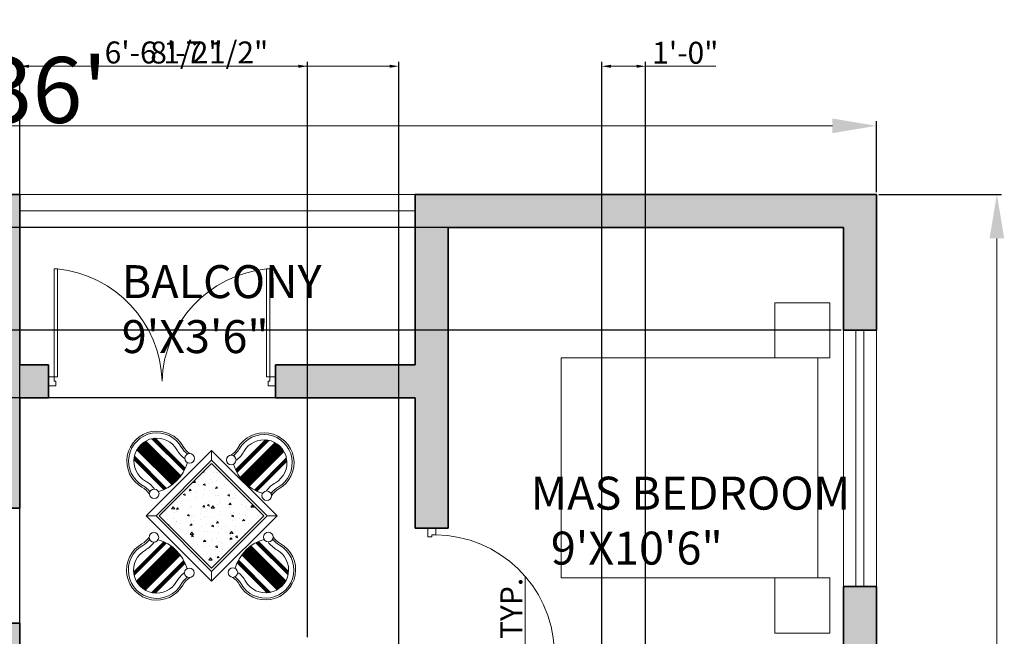
# Model space of a CAD drawing. Units: inches. Extents: x 2696 to 3240, y 1564 to 2310.
# Tile 76 of 76: x 2966 to 3235, y 2142 to 2310. Entities that reach past the tile are written whole.
import ezdxf

# ---------------------------------------------------------------- set-up
doc = ezdxf.new("R2010")
doc.units = ezdxf.units.IN
doc.linetypes.add('ACAD_ISO02W100', pattern=[15, 12, -3])
for name, color, linetype, lineweight in [('A-ANNO-DIMS', 3, 'Continuous', 18), ('A-AREA-IDEN', 7, 'Continuous', 18), ('A-DOOR', 4, 'Continuous', 18), ('A-FLOR-HRAL', 7, 'Continuous', 18), ('A-FURN', 251, 'Continuous', 13), ('A-WALL', 7, 'Continuous', 35), ('A-WALL-OVHD', 7, 'ACAD_ISO02W100', 18), ('A-WALL-PATT', 9, 'Continuous', 13), ('WINDOW', 2, 'Continuous', 18)]:
    doc.layers.add(name, color=color, linetype=linetype, lineweight=lineweight)
doc.styles.add('TIMES NEW', font='times.ttf')
doc.styles.add('YQ_DIM', font='SUPEROS.SHX', dxfattribs={"width": 0.8, "bigfont": 'HZDX.SHX'})
doc.dimstyles.new('Siddhuu', dxfattribs={"dimtxt": 6, "dimasz": 2.5, "dimexe": 1.25, "dimexo": 0.625, "dimtad": 1, "dimdec": 1, "dimlunit": 4, "dimtxsty": 'TIMES NEW', "dimcen": 2.5, "dimclrd": 256, "dimclre": 1, "dimclrt": 7, "dimadec": 0, "dimazin": 0, "dimtfac": 1, "dimtdec": 1, "dimtmove": 0, "dimatfit": 3, "dimfxl": 1, "dimtolj": 1, "dimlwd": -1, "dimarcsym": 0})

# ---------------------------------------------------------------- blocks, each defined once
blk = doc.blocks.new('DR_D01')
for p, q in [((-0.45, 0.93), (-0.42, 0.93)), ((-0.45, 0.03), (-0.45, 0.93)), ((-0.42, 0.03), (-0.42, 0.93)), ((-0.5, 0.03), (-0.42, 0.03)), ((-0.5, 0.03), (-0.5, -0.03)), ((-0.45, 0.03), (-0.45, 0)), ((-0.45, 0), (-0.435, 0)), ((-0.435, 0), (-0.435, -0.03)), ((0.435, 0), (0.435, -0.03)), ((0.45, 0), (0.435, 0)), ((0.45, 0.03), (0.45, 0)), ((0.5, 0.03), (0.45, 0.03)), ((0.5, -0.03), (0.5, 0.03)), ((-0.435, -0.03), (-0.5, -0.03)), ((0.435, -0.03), (0.5, -0.03))]:
    blk.add_line(p, q)
blk.add_arc((-0.4602, 0.0206), 0.9103, 0.59152, 87.46644)
blk = doc.blocks.new('DR_D02')
for p, q in [((-0.46, 0.4948), (-0.475, 0.4948)), ((-0.475, 0.02), (-0.475, 0.4948)), ((-0.46, 0.02), (-0.46, 0.495)), ((0.46, 0.02), (0.46, 0.495)), ((0.46, 0.4948), (0.475, 0.4948)), ((0.475, 0.02), (0.475, 0.4948)), ((-0.46, 0.02), (-0.5, 0.02)), ((-0.5, 0.02), (-0.5, -0.02)), ((-0.475, 0.02), (-0.475, 0)), ((-0.475, 0), (-0.4675, 0)), ((-0.4675, 0), (-0.4675, -0.02)), ((0.46, 0.02), (0.5, 0.02)), ((0.4675, 0), (0.4675, -0.02)), ((0.475, 0), (0.4675, 0)), ((0.475, 0.02), (0.475, 0)), ((0.5, 0.02), (0.5, -0.02)), ((-0.4675, -0.02), (-0.5, -0.02)), ((0.4675, -0.02), (0.5, -0.02))]:
    blk.add_line(p, q)
for centre, start, end in [((-0.5121, -0.0149), 1.6619, 84.1677), ((0.5121, -0.0149), 95.8323, 178.3381)]:
    blk.add_arc(centre, 0.5123, start, end)
blk = doc.blocks.new('WD_WIN4')
for p, q in [((-0.5, 0.5), (0.5, 0.5)), ((-0.5, 0.12), (0.5, 0.12)), ((-0.5, -0.12), (0.5, -0.12)), ((-0.5, -0.5), (0.5, -0.5))]:
    blk.add_line(p, q)
blk = doc.blocks.new('*D9')
at = {"layer": 'A-ANNO-DIMS', "color": 0, "lineweight": -2, "transparency": 16777216}
for p, q in [((2745.61, 2262.83), (2745.61, 2282.19)), ((3199.61, 2262.83), (3199.61, 2282.19))]:
    blk.add_line(p, q, dxfattribs=at)
at = {"layer": 'A-ANNO-DIMS', "color": 0, "transparency": 16777216}
blk.add_line((2757.61, 2280.94), (3187.61, 2280.94), dxfattribs=at)
for points in [[(2757.61, 2282.94), (2757.61, 2278.94), (2745.61, 2280.94)], [(3187.61, 2282.94), (3187.61, 2278.94), (3199.61, 2280.94)]]:
    blk.add_solid(points, dxfattribs=at)
at = {"layer": 'Defpoints', "color": 0, "transparency": 16777216}
for p in [(3199.61, 2280.94), (2745.61, 2262.2), (3199.61, 2262.2)]:
    blk.add_point(p, dxfattribs=at)
at = {"layer": 'A-ANNO-DIMS', "color": 0, "transparency": 16777216, "insert": (2972.61, 2290.72), "char_height": 18, "attachment_point": 5, "style": 'TIMES NEW'}
blk.add_mtext("\\A1;36'", dxfattribs=at)
blk = doc.blocks.new('*D10')
at = {"layer": 'A-ANNO-DIMS', "color": 0, "lineweight": -2, "transparency": 16777216}
for p, q in [((3200.24, 2262.2), (3233.75, 2262.2)), ((3200.24, 1605.2), (3233.75, 1605.2))]:
    blk.add_line(p, q, dxfattribs=at)
at = {"layer": 'A-ANNO-DIMS', "color": 0, "transparency": 16777216}
blk.add_line((3232.5, 2250.2), (3232.5, 1617.2), dxfattribs=at)
for points in [[(3230.5, 2250.2), (3234.5, 2250.2), (3232.5, 2262.2)], [(3230.5, 1617.2), (3234.5, 1617.2), (3232.5, 1605.2)]]:
    blk.add_solid(points, dxfattribs=at)
at = {"layer": 'Defpoints', "color": 0, "transparency": 16777216}
for p in [(3199.61, 2262.2), (3199.61, 1605.2), (3232.5, 1605.2)]:
    blk.add_point(p, dxfattribs=at)
at = {"layer": 'A-ANNO-DIMS', "color": 0, "transparency": 16777216, "insert": (3222.71, 1933.7), "char_height": 18, "attachment_point": 5, "rotation": 90, "style": 'TIMES NEW'}
blk.add_mtext("\\A1;54'", dxfattribs=at)
blk = doc.blocks.new('DINING-SET-4')
h = blk.add_hatch()
h.set_pattern_fill('AR-CONC,_O', color=256, scale=0.03156, angle=135)
h.set_pattern_definition([(185, (694.1166, -47.9622), (-3.709933, 4.421326), [0.60121, -6.613307]), (130, (694.1166, -47.962), (-3.47714, -5.050095), [0.48097, -5.290645]), (235.451, (693.8074, -47.594), (-7.187067, -0.628735), [0.51095, -5.620443]), (181.1842, (692.983, -49.096), (-5.11118, 6.98761), [0.90181, -9.91996]), (231.6356, (692.557, -48.514), (-10.81945, -0.22364), [0.76642, -8.43066]), (126.184, (692.983, -49.096), (-10.81945, -0.22362), [0.72145, -7.93597]), (156, (692.6995, -48.2457), (-1.10128, 5.66559), [0.60121, -6.613307]), (101, (692.6995, -48.2457), (-5.48951, -2.73116), [0.48097, -5.290645]), (206.4514, (692.608, -47.7735), (-6.590787, 2.93441), [0.51095, -5.620443]), (172.5, (694.1166, -47.9622), (-1.955854, -1.8180035), [0, -5.226516, 0, -5.370807, 0, -5.310686]), (142.5, (694.1166, -47.9622), (-3.726774, -0.744482), [0, -3.062161, 0, -5.106274, 0, -2.024073]), (102.5, (695.3806, -49.2263), (-2.8979947, 3.15368), [0, -2.004032, 0, -6.25258, 0, -8.296694]), (92.5, (695.9475, -49.793), (-3.873065, 2.73823), [0, -2.605242, 0, -4.152355, 0, -5.891855])])
h.paths.add_polyline_path([(23.22, 8.74), (37.5, 23.02), (23.22, 37.31), (8.94, 23.02)])
for p, q in [((14.34, 33.33), (4.62, 43.06)), ((14.5, 33.52), (4.82, 43.2)), ((14.65, 33.71), (5.03, 43.33)), ((14.79, 33.91), (5.25, 43.45)), ((15.69, 35.33), (6.93, 44.09)), ((15.81, 35.56), (7.22, 44.15)), ((15.92, 35.79), (7.52, 44.19)), ((16.03, 36.02), (7.83, 44.22)), ((29.77, 35.57), (37.97, 43.77)), ((29.88, 35.34), (38.28, 43.74)), ((29.99, 35.11), (38.58, 43.7)), ((30.11, 34.88), (38.86, 43.64)), ((12.42, 31.5), (2.84, 41.08)), ((12.61, 31.65), (2.97, 41.3)), ((12.8, 31.8), (3.1, 41.5)), ((12.99, 31.96), (3.24, 41.7)), ((13.17, 32.12), (3.39, 41.89)), ((13.35, 32.28), (3.55, 42.08)), ((13.52, 32.45), (3.71, 42.26)), ((13.69, 32.62), (3.88, 42.43)), ((13.86, 32.79), (4.05, 42.6)), ((14.03, 32.97), (4.24, 42.76)), ((14.19, 33.15), (4.42, 42.91)), ((23.22, 38.2), (23.22, 40.88)), ((31, 33.46), (40.55, 43.01)), ((31.15, 33.26), (40.76, 42.88)), ((31.3, 33.07), (40.97, 42.75)), ((31.45, 32.88), (41.18, 42.61)), ((31.61, 32.7), (41.37, 42.46)), ((31.77, 32.52), (41.56, 42.31)), ((31.93, 32.34), (41.74, 42.15)), ((32.1, 32.17), (41.92, 41.98)), ((32.27, 32), (42.09, 41.81)), ((32.45, 31.83), (42.25, 41.63)), ((32.63, 31.67), (42.4, 41.45)), ((32.81, 31.51), (42.55, 41.25)), ((32.99, 31.35), (42.69, 41.05)), ((33.18, 31.2), (42.83, 40.85)), ((33.38, 31.05), (42.96, 40.63)), ((10.21, 30.19), (2.02, 38.38)), ((10.44, 30.3), (2.05, 38.7)), ((10.67, 30.41), (2.09, 39)), ((10.9, 30.53), (2.15, 39.28)), ((34.9, 30.08), (43.65, 38.83)), ((35.12, 29.96), (43.7, 38.55)), ((35.35, 29.85), (43.75, 38.25)), ((35.58, 29.74), (43.78, 37.94)), ((8.05, 23.02), (5.37, 23.02)), ((38.4, 23.02), (41.07, 23.02)), ((10.15, 15.95), (1.95, 7.75)), ((10.38, 15.84), (1.98, 7.44)), ((10.61, 15.73), (2.02, 7.14)), ((10.84, 15.61), (2.08, 6.86)), ((12.26, 14.72), (2.71, 5.17)), ((12.46, 14.57), (2.84, 4.95)), ((12.65, 14.42), (2.97, 4.75)), ((12.83, 14.27), (3.11, 4.54)), ((13.02, 14.11), (3.26, 4.35)), ((13.2, 13.95), (3.41, 4.16)), ((13.38, 13.78), (3.57, 3.98)), ((13.55, 13.62), (3.74, 3.8)), ((13.72, 13.45), (3.91, 3.63)), ((32.44, 13.53), (42.25, 3.72)), ((32.61, 13.7), (42.42, 3.89)), ((32.78, 13.87), (42.59, 4.06)), ((32.96, 14.03), (42.75, 4.24)), ((33.14, 14.19), (42.9, 4.43)), ((33.33, 14.35), (43.05, 4.63)), ((33.51, 14.5), (43.19, 4.83)), ((33.7, 14.65), (43.32, 5.04)), ((33.9, 14.8), (43.45, 5.25)), ((35.33, 15.7), (44.08, 6.94)), ((35.55, 15.81), (44.14, 7.23)), ((35.78, 15.93), (44.18, 7.52)), ((36.01, 16.03), (44.21, 7.83)), ((13.89, 13.27), (4.09, 3.47)), ((14.05, 13.09), (4.27, 3.32)), ((14.21, 12.91), (4.47, 3.17)), ((14.36, 12.72), (4.67, 3.03)), ((14.52, 12.54), (4.87, 2.89)), ((14.67, 12.34), (5.08, 2.76)), ((15.64, 10.82), (6.89, 2.07)), ((30.52, 10.91), (39.27, 2.15)), ((31.49, 12.43), (41.08, 2.85)), ((31.64, 12.62), (41.29, 2.97)), ((31.8, 12.81), (41.5, 3.11)), ((31.95, 12.99), (41.69, 3.25)), ((32.11, 13.18), (41.89, 3.4)), ((32.27, 13.35), (42.07, 3.55)), ((15.75, 10.6), (7.17, 2.02)), ((15.87, 10.37), (7.47, 1.97)), ((15.98, 10.14), (7.78, 1.94)), ((30.18, 10.22), (38.38, 2.03)), ((30.29, 10.45), (38.69, 2.06)), ((30.41, 10.68), (38.99, 2.1)), ((23.22, 7.85), (23.22, 5.17))]:
    blk.add_line(p, q)
for points in [[(41.07, 23.02), (23.22, 40.88), (5.37, 23.02), (23.22, 5.17)], [(38.4, 23.02), (23.22, 38.2), (8.05, 23.02), (23.22, 7.85)], [(37.5, 23.02), (23.22, 37.31), (8.94, 23.02), (23.22, 8.74)]]:
    blk.add_lwpolyline(points, close=True)
for centre in [(17.23, 38.71), (28.57, 38.26), (7.55, 29.03), (38.27, 28.51), (7.46, 17.15), (38.7, 17.23), (17.14, 7.47), (29.03, 7.55)]:
    blk.add_circle(centre, 1.31)
for centre, radius, start, end in [((8.28, 37.96), 8.21, 29.1881, 240.1532), ((37.51, 37.51), 8.21, 299.8468, 150.8119), ((8.28, 37.96), 7.72, 29.1881, 240.1532), ((8.28, 37.96), 6.28, 29.2752, 240.1505), ((37.51, 37.51), 7.72, 299.8468, 150.8119), ((37.51, 37.51), 6.28, 299.8495, 150.7248), ((20.45, 44.88), 7.72, 209.8594, 234.0675), ((20.45, 44.88), 6.28, 210.1015, 232.6572), ((20.45, 44.88), 5.79, 210.1015, 236.9513), ((25.34, 44.43), 5.79, 303.0487, 329.8985), ((25.34, 44.43), 6.28, 307.3428, 329.8985), ((25.34, 44.43), 7.72, 305.9325, 330.1406), ((5.4, 40.81), 11.66, 286.5158, 343.8317), ((40.4, 40.36), 11.66, 196.1683, 253.4842), ((1.37, 25.79), 7.72, 36.1055, 60.6071), ((1.37, 25.79), 5.79, 32.6748, 60.7093), ((1.37, 25.79), 6.28, 37.2611, 60.7093), ((44.43, 25.34), 7.72, 119.3929, 143.8945), ((44.43, 25.34), 6.28, 119.2907, 142.7389), ((44.43, 25.34), 5.79, 119.2907, 147.3252), ((1.29, 20.38), 5.79, 300.1015, 326.9513), ((1.29, 20.38), 6.28, 300.1015, 322.6572), ((5.36, 5.32), 11.66, 16.5158, 73.8317), ((40.8, 5.4), 11.66, 106.1683, 163.4842), ((44.87, 20.46), 6.28, 217.3428, 239.8985), ((44.87, 20.46), 5.79, 213.0487, 239.8985), ((8.21, 8.21), 8.21, 119.1881, 330.1532), ((8.21, 8.21), 7.72, 119.1881, 330.1532), ((8.21, 8.21), 6.28, 119.2752, 330.1505), ((1.29, 20.38), 7.72, 299.8594, 324.0675), ((37.95, 8.29), 8.21, 209.8468, 60.8119), ((37.95, 8.29), 7.72, 209.8468, 60.8119), ((37.95, 8.29), 6.28, 209.8495, 60.7248), ((44.87, 20.46), 7.72, 215.9325, 240.1406), ((20.38, 1.29), 7.72, 126.1055, 150.6071), ((20.38, 1.29), 6.28, 127.2611, 150.7093), ((20.38, 1.29), 5.79, 122.6748, 150.7093), ((25.78, 1.37), 5.79, 29.2907, 57.3252), ((25.78, 1.37), 6.28, 29.2907, 52.7389), ((25.78, 1.37), 7.72, 29.3929, 53.8945)]:
    blk.add_arc(centre, radius, start, end)
blk = doc.blocks.new('BED-DOUBLE-WITH-NIGHTSTANDS')
for points in [[(0, 75.13), (0, 90.16), (15.03, 90.16), (15.03, 75.13)], [(3.28, 15.03), (3.28, 75.13), (73.4, 75.13), (73.4, 15.03)], [(0, 15.03), (0, 0), (15.03, 0), (15.03, 15.03)]]:
    blk.add_lwpolyline(points, close=True)
blk = doc.blocks.new('*D39')
at = {"layer": 'A-ANNO-DIMS', "transparency": 16777216}
for p, q in [((3103.69, 2104.03), (3103.69, 2157.84)), ((3103.69, 2091.94), (3103.69, 2101.53))]:
    blk.add_line(p, q, dxfattribs=at)
at = {"layer": 'A-ANNO-DIMS', "color": 1, "lineweight": -2, "transparency": 16777216}
for p, q in [((3105.99, 2104.03), (3102.44, 2104.03)), ((3105.99, 2089.44), (3102.44, 2089.44))]:
    blk.add_line(p, q, dxfattribs=at)
at = {"layer": 'A-ANNO-DIMS', "transparency": 16777216}
for points in [[(3103.28, 2101.53), (3104.11, 2101.53), (3103.69, 2104.03)], [(3103.28, 2091.94), (3104.11, 2091.94), (3103.69, 2089.44)]]:
    blk.add_solid(points, dxfattribs=at)
at = {"layer": 'Defpoints', "color": 0, "transparency": 16777216}
for p in [(3103.69, 2104.03), (3106.61, 2104.03), (3106.61, 2089.44)]:
    blk.add_point(p, dxfattribs=at)
at = {"layer": 'A-ANNO-DIMS', "color": 7, "transparency": 16777216, "insert": (3099.93, 2132.19), "char_height": 6, "attachment_point": 5, "rotation": 90, "style": 'TIMES NEW'}
blk.add_mtext('\\A1;1\'-2 1/2" TYP.', dxfattribs=at)
blk = doc.blocks.new('*D54')
at = {"layer": 'A-ANNO-DIMS', "color": 1, "lineweight": -2, "transparency": 16777216}
for p, q in [((3124.61, 1893.83), (3124.61, 2298.45)), ((3136.61, 1893.83), (3136.61, 2298.45))]:
    blk.add_line(p, q, dxfattribs=at)
at = {"layer": 'A-ANNO-DIMS', "transparency": 16777216}
for p, q in [((3127.11, 2297.2), (3134.11, 2297.2)), ((3136.61, 2297.2), (3155.76, 2297.2))]:
    blk.add_line(p, q, dxfattribs=at)
for points in [[(3127.11, 2297.62), (3127.11, 2296.78), (3124.61, 2297.2)], [(3134.11, 2297.62), (3134.11, 2296.78), (3136.61, 2297.2)]]:
    blk.add_solid(points, dxfattribs=at)
at = {"layer": 'Defpoints', "color": 0, "transparency": 16777216}
for p in [(3136.61, 2297.2), (3124.61, 1893.2), (3136.61, 1893.2)]:
    blk.add_point(p, dxfattribs=at)
at = {"layer": 'A-ANNO-DIMS', "color": 7, "transparency": 16777216, "insert": (3147.43, 2300.88), "char_height": 6, "attachment_point": 5, "style": 'TIMES NEW'}
blk.add_mtext('\\A1;1\'-0"', dxfattribs=at)
blk = doc.blocks.new('*D61')
at = {"layer": 'A-ANNO-DIMS', "color": 1, "lineweight": -2, "transparency": 16777216}
for p, q in [((2965.71, 2141.33), (2965.71, 2298.45)), ((3044.3, 2141.33), (3044.3, 2298.45))]:
    blk.add_line(p, q, dxfattribs=at)
at = {"layer": 'A-ANNO-DIMS', "transparency": 16777216}
blk.add_line((2968.21, 2297.2), (3041.8, 2297.2), dxfattribs=at)
for points in [[(2968.21, 2297.62), (2968.21, 2296.78), (2965.71, 2297.2)], [(3041.8, 2297.62), (3041.8, 2296.78), (3044.3, 2297.2)]]:
    blk.add_solid(points, dxfattribs=at)
at = {"layer": 'Defpoints', "color": 0, "transparency": 16777216}
for p in [(3044.3, 2297.2), (2965.71, 2140.7), (3044.3, 2140.7)]:
    blk.add_point(p, dxfattribs=at)
at = {"layer": 'A-ANNO-DIMS', "color": 7, "transparency": 16777216, "insert": (3005.01, 2300.96), "char_height": 6, "attachment_point": 5, "style": 'TIMES NEW'}
blk.add_mtext('\\A1;6\'-6 1/2"', dxfattribs=at)
blk = doc.blocks.new('*D63')
at = {"layer": 'A-ANNO-DIMS', "color": 1, "lineweight": -2, "transparency": 16777216}
for p, q in [((2965.71, 1989.83), (2965.71, 2298.45)), ((3069.21, 1989.83), (3069.21, 2298.45))]:
    blk.add_line(p, q, dxfattribs=at)
at = {"layer": 'A-ANNO-DIMS', "transparency": 16777216}
blk.add_line((2968.21, 2297.2), (3066.71, 2297.2), dxfattribs=at)
for points in [[(2968.21, 2297.62), (2968.21, 2296.78), (2965.71, 2297.2)], [(3066.71, 2297.62), (3066.71, 2296.78), (3069.21, 2297.2)]]:
    blk.add_solid(points, dxfattribs=at)
at = {"layer": 'Defpoints', "color": 0, "transparency": 16777216}
for p in [(3069.21, 2297.2), (2965.71, 1989.2), (3069.21, 1989.2)]:
    blk.add_point(p, dxfattribs=at)
at = {"layer": 'A-ANNO-DIMS', "color": 7, "transparency": 16777216, "insert": (3017.46, 2300.96), "char_height": 6, "attachment_point": 5, "style": 'TIMES NEW'}
blk.add_mtext('\\A1;8\'-7 1/2"', dxfattribs=at)
blk = doc.blocks.new('*D64')
at = {"layer": 'A-ANNO-DIMS', "color": 1, "lineweight": -2, "transparency": 16777216}
for p, q in [((3073.08, 2206.7), (2709.36, 2206.7)), ((3068.58, 1989.2), (2709.36, 1989.2))]:
    blk.add_line(p, q, dxfattribs=at)
at = {"layer": 'A-ANNO-DIMS', "transparency": 16777216}
blk.add_line((2710.61, 1991.7), (2710.61, 2204.2), dxfattribs=at)
for points in [[(2710.19, 2204.2), (2711.03, 2204.2), (2710.61, 2206.7)], [(2710.19, 1991.7), (2711.03, 1991.7), (2710.61, 1989.2)]]:
    blk.add_solid(points, dxfattribs=at)
at = {"layer": 'Defpoints', "color": 0, "transparency": 16777216}
for p in [(2710.61, 2206.7), (3073.71, 2206.7), (3069.21, 1989.2)]:
    blk.add_point(p, dxfattribs=at)
at = {"layer": 'A-ANNO-DIMS', "color": 7, "transparency": 16777216, "insert": (2706.85, 2097.95), "char_height": 6, "attachment_point": 5, "rotation": 90, "style": 'TIMES NEW'}
blk.add_mtext('\\A1;18\'-1 1/2"', dxfattribs=at)
blk = doc.blocks.new('*D76')
at = {"layer": 'A-ANNO-DIMS', "color": 1, "lineweight": -2, "transparency": 16777216}
for p, q in [((3189.99, 2253.2), (2709.36, 2253.2)), ((3189.99, 2225.2), (2709.36, 2225.2))]:
    blk.add_line(p, q, dxfattribs=at)
at = {"layer": 'A-ANNO-DIMS', "transparency": 16777216}
blk.add_line((2710.61, 2250.7), (2710.61, 2227.7), dxfattribs=at)
for points in [[(2710.19, 2250.7), (2711.03, 2250.7), (2710.61, 2253.2)], [(2710.19, 2227.7), (2711.03, 2227.7), (2710.61, 2225.2)]]:
    blk.add_solid(points, dxfattribs=at)
at = {"layer": 'Defpoints', "color": 0, "transparency": 16777216}
for p in [(3190.61, 2253.2), (2710.61, 2225.2), (3190.61, 2225.2)]:
    blk.add_point(p, dxfattribs=at)
at = {"layer": 'A-ANNO-DIMS', "color": 7, "transparency": 16777216, "insert": (2706.99, 2239.2), "char_height": 6, "attachment_point": 5, "rotation": 90, "style": 'TIMES NEW'}
blk.add_mtext('\\A1;2\'-4"', dxfattribs=at)

msp = doc.modelspace()

# ---------------------------------------------------------------- hatches: boundary and pattern name
at = {"layer": 'A-WALL-PATT', "transparency": 33554556}
h = msp.add_hatch(color=256, dxfattribs=at)
h.dxf.hatch_style = 1
h.paths.add_polyline_path([(2879.11, 2253.2), (2905.91, 2253.2), (2905.91, 2262.2), (2841.89, 2262.2), (2841.89, 2253.2), (2870.11, 2253.2), (2870.11, 2176.6), (2965.71, 2176.6), (2965.71, 2206.7), (2973.58, 2206.7), (2973.58, 2215.7), (2965.71, 2215.7), (2965.71, 2262.2), (2929.91, 2262.2), (2929.91, 2253.2), (2956.71, 2253.2), (2956.71, 2185.6), (2879.11, 2185.6)])
h.paths.add_polyline_path([(2782.83, 2262.2), (2745.61, 2262.2), (2745.61, 2228.73), (2754.61, 2228.73), (2754.61, 2253.2), (2782.83, 2253.2)])
h.paths.add_polyline_path([(2754.61, 2136.2), (2965.71, 2136.2), (2965.71, 2145.2), (2879.11, 2145.2), (2879.11, 2147.07), (2877.34, 2147.07), (2870.11, 2147.07), (2870.11, 2145.2), (2754.61, 2145.2), (2754.61, 2169.67), (2745.61, 2169.67), (2745.61, 2000.2), (2754.61, 2000.2), (2754.61, 2019.2), (2849.08, 2019.2), (2849.08, 2023.7), (2841.21, 2023.7), (2841.21, 2051.83), (2836.71, 2051.83), (2836.71, 2023.7), (2754.61, 2023.7), (2754.61, 2091.2), (2836.71, 2091.2), (2836.71, 2087.83), (2841.21, 2087.83), (2841.21, 2095.7), (2754.61, 2095.7)])
h.paths.add_polyline_path([(2965.71, 2136.2), (2956.71, 2136.2), (2956.71, 2023.7), (2885.08, 2023.7), (2885.08, 2019.2), (2956.71, 2019.2), (2956.71, 1950.58), (2965.71, 1950.58), (2965.71, 1980.2), (2973.58, 1980.2), (2973.58, 1989.2), (2965.71, 1989.2)])
h.paths.add_polyline_path([(2754.61, 1906.7), (2880.21, 1906.7), (2884.71, 1906.7), (2956.71, 1906.7), (2956.71, 1792.7), (2944.71, 1792.7), (2944.71, 1783.7), (2956.71, 1783.7), (2956.71, 1740.2), (2884.71, 1740.2), (2884.71, 1783.7), (2896.71, 1783.7), (2896.71, 1792.7), (2884.71, 1792.7), (2884.71, 1846.7), (2880.21, 1846.7), (2880.21, 1740.2), (2754.61, 1740.2), (2754.61, 1777.2), (2745.61, 1777.2), (2745.61, 1692.7), (2754.61, 1692.7), (2754.61, 1731.2), (2956.71, 1731.2), (2956.71, 1723.33), (2965.71, 1723.33), (2965.71, 1884.2), (2973.58, 1884.2), (2973.58, 1893.2), (2965.71, 1893.2), (2965.71, 1914.58), (2956.71, 1914.58), (2956.71, 1911.2), (2754.61, 1911.2), (2754.61, 1930.2), (2745.61, 1930.2), (2745.61, 1817.2), (2754.61, 1817.2), (2754.61, 1854.2), (2826.61, 1854.2), (2826.61, 1868.83), (2822.11, 1868.83), (2822.11, 1858.7), (2754.61, 1858.7)])
h.paths.add_polyline_path([(2965.71, 1656.2), (3008.24, 1656.2), (3008.24, 1665.2), (2965.71, 1665.2), (2965.71, 1693.33), (2956.71, 1693.33), (2956.71, 1686.2), (2934.58, 1686.2), (2934.58, 1681.7), (2956.71, 1681.7), (2956.71, 1614.2), (2896.71, 1614.2), (2896.71, 1681.7), (2904.58, 1681.7), (2904.58, 1686.2), (2892.21, 1686.2), (2892.21, 1614.2), (2858.41, 1614.2), (2858.41, 1605.2), (2965.71, 1605.2)])
h.paths.add_polyline_path([(2788.41, 1614.2), (2754.61, 1614.2), (2754.61, 1652.7), (2745.61, 1652.7), (2745.61, 1605.2), (2788.41, 1605.2)])
h.paths.add_polyline_path([(3199.61, 1633.05), (3190.61, 1633.05), (3190.61, 1614.2), (3082.61, 1614.2), (3082.61, 1665.2), (3070.24, 1665.2), (3070.24, 1656.2), (3078.11, 1656.2), (3078.11, 1605.2), (3199.61, 1605.2)])
h.paths.add_polyline_path([(3199.61, 1702.05), (3190.61, 1702.05), (3190.61, 1699.7), (3106.61, 1699.7), (3106.61, 1747.7), (3190.61, 1747.7), (3190.61, 1752.2), (3082.61, 1752.2), (3082.61, 1760.08), (3078.11, 1760.08), (3078.11, 1747.7), (3102.11, 1747.7), (3102.11, 1699.7), (3078.11, 1699.7), (3078.11, 1695.2), (3190.61, 1695.2), (3190.61, 1676.35), (3199.61, 1676.35)])
h.paths.add_polyline_path([(3199.61, 1783.2), (3190.61, 1783.2), (3190.61, 1745.35), (3199.61, 1745.35)])
h.paths.add_polyline_path([(3082.61, 1884.2), (3190.61, 1884.2), (3190.61, 1853.2), (3199.61, 1853.2), (3199.61, 1901.7), (3190.61, 1901.7), (3190.61, 1893.2), (3005.58, 1893.2), (3005.58, 1891.28), (3005.58, 1884.2), (3078.11, 1884.2), (3078.11, 1792.08), (3082.61, 1792.08)])
h.paths.add_polyline_path([(3199.61, 1994.7), (3190.61, 1994.7), (3190.61, 1989.2), (3073.71, 1989.2), (3073.71, 2034.2), (3069.21, 2034.2), (3069.21, 1989.2), (3005.58, 1989.2), (3005.58, 1980.2), (3190.61, 1980.2), (3190.61, 1971.7), (3199.61, 1971.7)])
h.paths.add_polyline_path([(3199.61, 2155.2), (3190.61, 2155.2), (3190.61, 2064.7), (3199.61, 2064.7)])
h.paths.add_polyline_path([(3190.61, 2074.7), (3106.61, 2074.7), (3106.61, 2122.7), (3190.61, 2122.7), (3190.61, 2127.2), (3082.71, 2127.2), (3082.71, 2135.08), (3073.71, 2135.08), (3073.71, 2122.7), (3102.11, 2122.7), (3102.11, 2074.7), (3069.21, 2074.7), (3069.21, 2070.2), (3190.61, 2070.2)])
h.paths.add_polyline_path([(3082.71, 2253.2), (3190.61, 2253.2), (3190.61, 2225.2), (3199.61, 2225.2), (3199.61, 2262.2), (3073.71, 2262.2), (3073.71, 2215.7), (3035.58, 2215.7), (3035.58, 2206.7), (3073.71, 2206.7), (3073.71, 2171.08), (3082.71, 2171.08)])

# ---------------------------------------------------------------- linework, layer by layer
at = {"layer": 'A-FLOR-HRAL'}
for p, q in [((3073.71, 2262.2), (2965.71, 2262.2)), ((3073.71, 2257.7), (2965.71, 2257.7))]:
    msp.add_line(p, q, dxfattribs=at)
at = {"layer": 'A-WALL'}
for p, q in [((2929.91, 2262.2), (2965.71, 2262.2)), ((2965.71, 2215.7), (2965.71, 2262.2)), ((3073.71, 2262.2), (3199.61, 2262.2)), ((3073.71, 2215.7), (3073.71, 2262.2)), ((3199.61, 2225.2), (3199.61, 2262.2)), ((3082.71, 2253.2), (3190.61, 2253.2)), ((3082.71, 2171.08), (3082.71, 2253.2)), ((3190.61, 2225.2), (3190.61, 2253.2)), ((3190.61, 2225.2), (3199.61, 2225.2)), ((2973.58, 2215.7), (2965.71, 2215.7)), ((2973.58, 2206.7), (2973.58, 2215.7)), ((3073.71, 2215.7), (3035.58, 2215.7)), ((3035.58, 2206.7), (3035.58, 2215.7)), ((2965.71, 2176.6), (2965.71, 2206.7)), ((2973.58, 2206.7), (2965.71, 2206.7)), ((3073.71, 2206.7), (3035.58, 2206.7)), ((3073.71, 2171.08), (3073.71, 2206.7)), ((2870.11, 2176.6), (2965.71, 2176.6)), ((3082.71, 2171.08), (3073.71, 2171.08)), ((3190.61, 2155.2), (3199.61, 2155.2)), ((3190.61, 2064.7), (3190.61, 2155.2)), ((3199.61, 2064.7), (3199.61, 2155.2)), ((2879.11, 2145.2), (2965.71, 2145.2)), ((2965.71, 2145.2), (2965.71, 2136.2))]:
    msp.add_line(p, q, dxfattribs=at)
at = {"layer": 'A-WALL-OVHD'}
msp.add_line((2965.71, 2176.6), (2965.71, 2145.2), dxfattribs=at)

# ---------------------------------------------------------------- block references
at = {"layer": 'A-DOOR', "xscale": -62, "yscale": 62, "zscale": 62}
msp.add_blockref('DR_D02', (3004.58, 2211.2), dxfattribs=at)
at = {"layer": 'A-DOOR', "xscale": 36, "yscale": -36, "zscale": 36, "rotation": 90}
msp.add_blockref('DR_D01', (3078.21, 2153.08), dxfattribs=at)
at = {"layer": 'A-FURN', "rotation": 180}
msp.add_blockref('BED-DOUBLE-WITH-NIGHTSTANDS', (3186.92, 2232.65), dxfattribs=at)
at = {"layer": 'A-FURN'}
msp.add_blockref('DINING-SET-4', (2994.89, 2151.45), dxfattribs=at)
at = {"layer": 'WINDOW', "xscale": 70, "yscale": 8.999999999999545, "zscale": 70, "rotation": 270}
msp.add_blockref('WD_WIN4', (3195.11, 2190.2), dxfattribs=at)

# ---------------------------------------------------------------- texts
at = {"layer": 'A-AREA-IDEN', "char_height": 9, "attachment_point": 1, "style": 'YQ_DIM'}
for s, width, insert in [('BALCONY\\P9\'X3\'6"', 48.0032, (2993.57, 2242.91)), ('MAS BEDROOM\\P  9\'X10\'6"', 92.6128, (3105.22, 2185.17))]:
    msp.add_mtext_dynamic_manual_height_columns(s, width=width, gutter_width=12.5, heights=[0], dxfattribs=dict(at, insert=insert))

# ---------------------------------------------------------------- dimensions: what is measured, and where the dimension line sits
at = {"layer": 'A-ANNO-DIMS'}
for base, p1, p2, picture, middle in [((3044.3, 2297.2), (2965.71, 2140.7), (3044.3, 2140.7), '*D61', (3005.01, 2300.96)), ((3069.21, 2297.2), (2965.71, 1989.2), (3069.21, 1989.2), '*D63', (3017.46, 2300.96)), ((3136.61, 2297.2), (3124.61, 1893.2), (3136.61, 1893.2), '*D54', (3147.43, 2300.88))]:
    dim = msp.add_linear_dim(base=base, p1=p1, p2=p2, dimstyle='Siddhuu', override={"dimdec": 1, "dimlfac": 1, "dimrnd": 0, "dimzin": 1, "dimdsep": 46, "dimlunit": 4, "dimfrac": 2}, dxfattribs=at)
    dim.commit()
    dim.dimension.update_dxf_attribs({"geometry": picture, "text_midpoint": middle})
dim = msp.add_linear_dim(base=(3199.61, 2280.94), p1=(2745.61, 2262.2), p2=(3199.61, 2262.2), text="36'", dimstyle='Siddhuu', override={"dimtxt": 18, "dimasz": 12, "dimclrd": 0, "dimclre": 0, "dimclrt": 0}, dxfattribs=at)
dim.commit()
dim.dimension.update_dxf_attribs({"geometry": '*D9', "text_midpoint": (2972.61, 2290.72)})
for base, p1, p2, text, override, picture, middle in [((3232.5, 1605.2), (3199.61, 2262.2), (3199.61, 1605.2), "54'", {"dimtxt": 18, "dimasz": 12, "dimclrd": 0, "dimclre": 0, "dimclrt": 0}, '*D10', (3222.71, 1933.7)), ((3103.69, 2104.03), (3106.61, 2089.44), (3106.61, 2104.03), '<> TYP.', {"dimdec": 1, "dimlfac": 1, "dimrnd": 0, "dimzin": 1, "dimdsep": 46, "dimlunit": 4, "dimfrac": 2}, '*D39', (3099.93, 2132.19))]:
    dim = msp.add_linear_dim(base=base, p1=p1, p2=p2, angle=90, text=text, dimstyle='Siddhuu', override=override, dxfattribs=at)
    dim.commit()
    dim.dimension.update_dxf_attribs({"geometry": picture, "text_midpoint": middle})
for base, p1, p2, picture, middle in [((2710.61, 2225.2), (3190.61, 2253.2), (3190.61, 2225.2), '*D76', (2706.99, 2239.2)), ((2710.61, 2206.7), (3069.21, 1989.2), (3073.71, 2206.7), '*D64', (2706.85, 2097.95))]:
    dim = msp.add_linear_dim(base=base, p1=p1, p2=p2, angle=90, dimstyle='Siddhuu', override={"dimdec": 1, "dimlfac": 1, "dimrnd": 0, "dimzin": 1, "dimdsep": 46, "dimlunit": 4, "dimfrac": 2}, dxfattribs=at)
    dim.commit()
    dim.dimension.update_dxf_attribs({"geometry": picture, "text_midpoint": middle})

doc.saveas('drawing.dxf')
